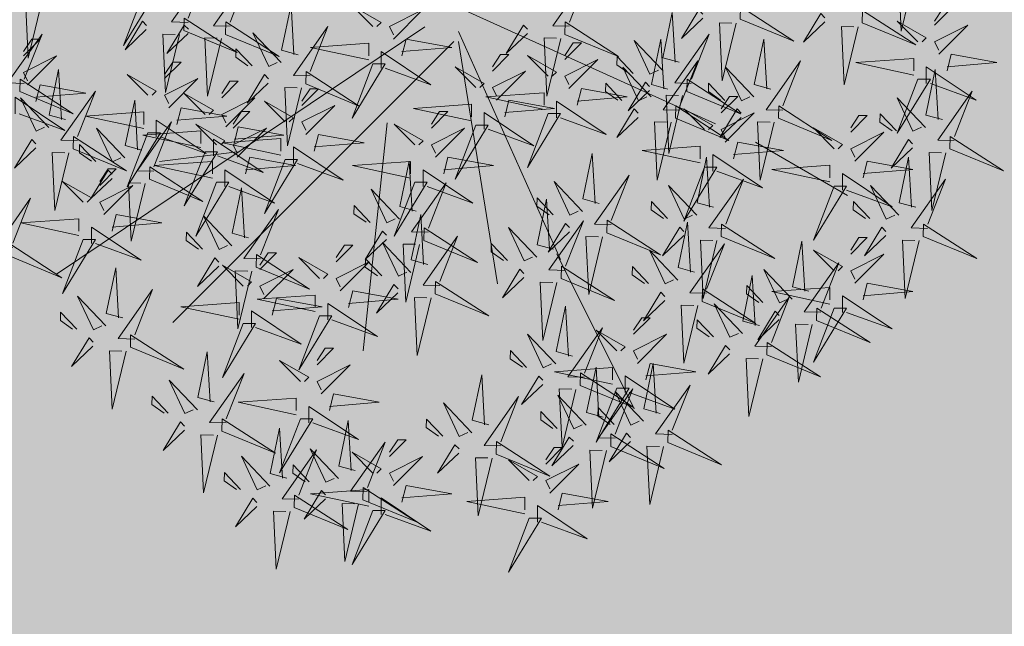
# Model space of a CAD drawing. Units: inches. Extents: x 1704 to 6393, y -157 to 1172.
# Tile 108 of 122: x 2688 to 2716, y 972 to 989. Entities that reach past the tile are written whole.
import ezdxf

# ---------------------------------------------------------------- set-up
doc = ezdxf.new("R2010")
doc.units = ezdxf.units.IN
doc.header["$MEASUREMENT"] = 0
doc.layers.add('A-ANNO-DIMS', color=7, linetype='Continuous', lineweight=13)
doc.layers.add('L-shrub', color=74, linetype='Continuous', lineweight=18)
doc.layers.add('L-HRDS-PATT', color=9, linetype='Continuous', lineweight=13, true_color=0xc5c1ba)
doc.styles.get("Standard").update_dxf_attribs({"font": 'arial.ttf'})
doc.dimstyles.get("Standard").update_dxf_attribs({"dimtxt": 6, "dimasz": 2, "dimexe": 0.18, "dimexo": 0.0625, "dimgap": 0.09, "dimtad": 0, "dimtih": 1, "dimtoh": 1, "dimdec": 1, "dimzin": 0, "dimdsep": 46, "dimlunit": 3, "dimtxsty": 'Standard', "dimblk": 'ARCHTICK', "dimcen": 0.09, "dimadec": 0, "dimazin": 0, "dimtfac": 1, "dimtdec": 1, "dimtofl": 0, "dimtmove": 0, "dimatfit": 3, "dimfxl": 1, "dimtolj": 1, "dimtzin": 0, "dimarcsym": 0})

# ---------------------------------------------------------------- blocks, each defined once
blk = doc.blocks.new('shrub3')
for p, q in [((68.94, 162.35), (98.58, 213.48)), ((-5.99, -2.5), (58.67, 140.12)), ((130.91, 52.02), (217.13, 95.08)), ((7.48, -2.5), (134.11, 54.01)), ((12.87, -2.5), (147.58, 19.03)), ((12.87, -5.19), (169.14, -161.27)), ((4.78, -21.34), (142.19, -225.85)), ((58.17, -42.16), (184.8, -55.61)), ((74.33, -125.58), (79.72, -168.64))]:
    blk.add_line(p, q)
for points in [[(29.32, 268.76), (20.08, 271.07), (24.7, 296.43), (27.01, 268.76)], [(72.58, 270.39), (84.86, 300.11), (65.67, 270.57), (72.58, 270.39)], [(36.24, 257.23), (27.01, 257.23), (45.48, 284.9), (36.24, 259.54)], [(121.34, 255.57), (133.62, 285.29), (114.43, 255.75), (121.34, 255.57)], [(20.08, 264.15), (3.92, 280.29), (13.16, 261.85), (17.78, 264.15)], [(68.03, 272.82), (67.8, 263.59), (40.6, 282.74), (65.73, 272.87)], [(3.92, 261.85), (-5.31, 271.07), (-5.31, 266.46), (1.62, 261.85)], [(74.83, 268.03), (106.93, 260.3), (74.6, 258.8), (74.77, 265.72)], [(56.33, 266.18), (53.8, 257.01), (28.56, 262.26), (56.27, 263.87)], [(116.79, 258), (116.56, 248.76), (89.36, 267.92), (114.49, 258.05)], [(13.16, 252.62), (1.62, 241.09), (10.85, 257.23), (13.16, 254.93)], [(33.94, 252.62), (63.95, 241.09), (33.94, 259.54), (33.94, 252.62)], [(60.71, 256.84), (44.17, 241.08), (62.84, 249.85), (60.65, 254.53)], [(123.59, 253.21), (155.69, 245.48), (123.36, 243.97), (123.53, 250.9)], [(-24.81, 251.09), (7.29, 243.36), (-25.04, 241.86), (-24.87, 248.78)], [(2.62, 221.69), (14.9, 251.41), (-4.29, 221.87), (2.62, 221.69)], [(31.63, 250.32), (24.7, 218.04), (22.39, 250.32), (29.32, 250.32)], [(72.06, 249.62), (83.3, 237.79), (67.4, 247.43), (69.76, 249.68)], [(105.09, 251.36), (102.56, 242.19), (77.32, 247.44), (105.04, 249.05)], [(88.68, 222.18), (79.44, 224.49), (84.06, 249.85), (86.37, 222.18)], [(156.52, 222.18), (147.29, 224.49), (151.9, 249.85), (154.21, 222.18)], [(109.47, 242.01), (92.93, 226.26), (111.6, 235.03), (109.41, 239.71)], [(62.61, 240.62), (53.16, 231.62), (57.77, 231.51), (62.55, 238.31)], [(95.61, 210.65), (86.37, 210.65), (104.84, 238.32), (95.61, 212.96)], [(163.45, 210.65), (154.21, 210.65), (172.68, 238.32), (163.45, 212.96)], [(79.44, 217.57), (63.28, 233.71), (72.52, 215.26), (77.14, 217.57)], [(120.82, 234.8), (132.06, 222.97), (116.16, 232.61), (118.52, 234.86)], [(147.29, 217.57), (131.13, 233.71), (140.36, 215.26), (144.98, 217.57)], [(63.28, 215.26), (54.05, 224.49), (54.05, 219.87), (60.98, 215.26)], [(111.37, 225.8), (101.92, 216.8), (106.53, 216.68), (111.31, 223.49)], [(131.13, 215.26), (121.89, 224.49), (121.89, 219.87), (128.82, 215.26)], [(167.98, 196.29), (180.26, 226), (161.07, 196.46), (167.98, 196.29)], [(4.87, 219.33), (36.97, 211.6), (4.64, 210.1), (4.81, 217.02)], [(72.52, 206.04), (60.98, 194.51), (70.21, 210.65), (72.52, 208.35)], [(93.3, 206.04), (123.31, 194.51), (93.3, 212.96), (93.3, 206.04)], [(140.36, 206.04), (128.82, 194.51), (138.05, 210.65), (140.36, 208.35)], [(163.43, 198.71), (163.2, 189.48), (136, 208.63), (161.13, 198.77)], [(161.14, 206.04), (191.15, 194.51), (161.14, 212.96), (161.14, 206.04)], [(55.62, 175.11), (67.9, 204.83), (48.71, 175.28), (55.62, 175.11)], [(90.99, 203.73), (84.06, 171.45), (81.75, 203.73), (88.68, 203.73)], [(158.83, 203.73), (151.9, 171.45), (149.59, 203.73), (156.52, 203.73)], [(2.1, 200.92), (13.34, 189.09), (-2.56, 198.73), (-0.2, 200.98)], [(187.06, 168.76), (199.34, 198.47), (180.15, 168.93), (187.06, 168.76)], [(151.73, 192.07), (149.2, 182.9), (123.96, 188.15), (151.68, 189.77)], [(170.23, 193.92), (202.33, 186.19), (170, 184.69), (170.17, 191.61)], [(51.07, 177.53), (50.84, 168.3), (23.64, 187.46), (48.77, 177.59)], [(0.5, 153.94), (12.78, 183.65), (-6.41, 154.11), (0.5, 153.94)], [(156.11, 182.73), (139.57, 166.97), (158.24, 175.74), (156.05, 180.42)], [(182.51, 171.18), (182.28, 161.95), (155.08, 181.11), (180.21, 171.24)], [(78.08, 150.19), (68.84, 152.49), (73.46, 177.86), (75.77, 150.19)], [(167.46, 175.51), (178.7, 163.69), (162.8, 173.32), (165.16, 175.57)], [(39.37, 170.9), (36.84, 161.73), (11.6, 166.98), (39.31, 168.59)], [(57.87, 172.75), (89.97, 165.01), (57.64, 163.51), (57.81, 170.44)], [(121.34, 143.35), (133.62, 173.06), (114.43, 143.52), (121.34, 143.35)], [(85.01, 138.66), (75.77, 138.66), (94.24, 166.33), (85.01, 140.97)], [(170.81, 164.55), (168.28, 155.37), (143.04, 160.62), (170.76, 162.24)], [(158.01, 166.51), (148.56, 157.51), (153.17, 157.4), (157.96, 164.21)], [(189.31, 166.39), (221.41, 158.66), (189.08, 157.16), (189.25, 164.09)], [(43.75, 161.55), (27.21, 145.8), (45.88, 154.57), (43.69, 159.24)], [(68.84, 145.58), (52.68, 161.72), (61.92, 143.27), (66.54, 145.58)], [(157.38, 132.76), (169.66, 162.48), (150.47, 132.94), (157.38, 132.76)], [(40.78, 124.29), (53.06, 154.01), (33.87, 124.47), (40.78, 124.29)], [(55.1, 154.34), (66.34, 142.51), (50.44, 152.15), (52.8, 154.4)], [(116.79, 145.77), (116.56, 136.54), (89.36, 155.7), (114.49, 145.83)], [(175.19, 155.2), (158.65, 139.45), (177.32, 148.22), (175.13, 152.89)], [(2.75, 151.57), (34.85, 143.84), (2.52, 142.34), (2.69, 149.26)], [(52.68, 143.27), (43.45, 152.49), (43.45, 147.88), (50.38, 143.27)], [(186.54, 147.99), (197.78, 136.16), (181.88, 145.8), (184.24, 148.05)], [(45.65, 145.34), (36.2, 136.34), (40.81, 136.22), (45.59, 143.03)], [(55.62, 117.94), (67.9, 147.66), (48.71, 118.11), (55.62, 117.94)], [(152.83, 135.19), (152.6, 125.95), (125.4, 145.11), (150.53, 135.24)], [(235.82, 113.71), (248.1, 143.42), (228.91, 113.88), (235.82, 113.71)], [(61.92, 134.05), (50.38, 122.52), (59.61, 138.66), (61.92, 136.35)], [(105.09, 139.14), (102.56, 129.96), (77.32, 135.21), (105.04, 136.83)], [(82.7, 134.05), (112.71, 122.52), (82.7, 140.97), (82.7, 134.05)], [(123.59, 140.98), (155.69, 133.25), (123.36, 131.75), (123.53, 138.68)], [(177.09, 138.99), (167.64, 129.99), (172.25, 129.87), (177.04, 136.68)], [(-0.02, 133.17), (11.22, 121.34), (-4.68, 130.97), (-2.32, 133.22)], [(36.23, 126.72), (36, 117.49), (8.8, 136.64), (33.93, 126.77)], [(80.39, 131.74), (73.46, 99.46), (71.15, 131.74), (78.08, 131.74)], [(51.07, 120.36), (50.84, 111.13), (23.64, 130.29), (48.77, 120.42)], [(109.47, 129.79), (92.93, 114.04), (111.6, 122.81), (109.41, 127.48)], [(141.13, 128.55), (138.6, 119.38), (113.36, 124.63), (141.08, 126.24)], [(159.63, 130.4), (191.73, 122.67), (159.4, 121.17), (159.57, 128.09)], [(201.04, 101.49), (191.81, 103.79), (196.42, 129.16), (198.73, 101.49)], [(231.27, 116.13), (231.04, 106.9), (203.84, 126.05), (228.97, 116.19)], [(43.03, 121.93), (75.13, 114.2), (42.8, 112.7), (42.97, 119.62)], [(120.82, 122.58), (132.06, 110.75), (116.16, 120.39), (118.52, 122.64)], [(24.53, 120.08), (22, 110.91), (-3.24, 116.16), (24.47, 117.77)], [(57.87, 115.58), (89.97, 107.84), (57.64, 106.34), (57.81, 113.27)], [(145.51, 119.2), (128.97, 103.45), (147.64, 112.22), (145.45, 116.9)], [(207.97, 89.96), (198.73, 89.96), (217.2, 117.63), (207.97, 92.27)], [(39.37, 113.73), (36.84, 104.56), (11.6, 109.81), (39.31, 111.42)], [(28.91, 110.73), (12.37, 94.98), (31.04, 103.75), (28.85, 108.43)], [(111.37, 113.58), (101.92, 104.58), (106.53, 104.46), (111.31, 111.27)], [(119.22, 79.83), (131.5, 109.54), (112.31, 80), (119.22, 79.83)], [(156.86, 111.99), (168.1, 100.16), (152.2, 109.8), (154.56, 112.05)], [(191.81, 96.88), (175.65, 113.02), (184.88, 94.57), (189.5, 96.88)], [(219.57, 109.49), (217.04, 100.32), (191.8, 105.57), (219.52, 107.19)], [(237.94, 81.95), (250.22, 111.66), (231.03, 82.12), (237.94, 81.95)], [(238.07, 111.34), (270.17, 103.61), (237.84, 102.11), (238.01, 109.03)], [(43.75, 104.38), (27.21, 88.63), (45.88, 97.4), (43.69, 102.07)], [(40.26, 103.52), (51.5, 91.69), (35.6, 101.33), (37.96, 103.58)], [(147.41, 102.99), (137.96, 93.99), (142.57, 93.88), (147.36, 100.68)], [(175.65, 94.57), (166.41, 103.79), (166.41, 99.18), (173.34, 94.57)], [(223.95, 100.15), (207.41, 84.4), (226.08, 93.17), (223.89, 97.84)], [(30.81, 94.52), (21.36, 85.52), (25.97, 85.41), (30.75, 92.21)], [(55.1, 97.17), (66.34, 85.34), (50.44, 94.98), (52.8, 97.23)], [(204.02, 65.01), (216.3, 94.72), (197.11, 65.18), (204.02, 65.01)], [(233.39, 84.37), (233.16, 75.14), (205.96, 94.29), (231.09, 84.43)], [(235.3, 92.94), (246.54, 81.11), (230.64, 90.74), (233, 92.99)], [(45.65, 88.17), (36.2, 79.17), (40.81, 79.05), (45.59, 85.86)], [(48.4, 63.38), (39.16, 65.68), (43.78, 91.04), (46.09, 63.38)], [(114.67, 82.25), (114.44, 73.02), (87.24, 92.18), (112.37, 82.31)], [(184.88, 85.35), (173.34, 73.82), (182.57, 89.96), (184.88, 87.65)], [(205.66, 85.35), (235.67, 73.82), (205.66, 92.27), (205.66, 85.35)], [(8.98, 56.54), (21.26, 86.25), (2.07, 56.71), (8.98, 56.54)], [(144.66, 54.42), (156.94, 84.13), (137.75, 54.59), (144.66, 54.42)], [(203.35, 83.04), (196.42, 50.76), (194.11, 83.04), (201.04, 83.04)], [(225.85, 83.93), (216.4, 74.93), (221.01, 74.82), (225.8, 81.63)], [(55.33, 51.85), (46.09, 51.85), (64.56, 79.52), (55.33, 54.15)], [(121.47, 77.46), (153.57, 69.73), (121.24, 68.23), (121.41, 75.15)], [(199.47, 67.43), (199.24, 58.2), (172.04, 77.35), (197.17, 67.49)], [(221.69, 77.73), (219.16, 68.56), (193.92, 73.81), (221.64, 75.43)], [(240.19, 79.58), (272.29, 71.85), (239.96, 70.35), (240.13, 77.27)], [(273.12, 52.79), (263.89, 55.09), (268.5, 80.46), (270.81, 52.79)], [(39.16, 58.76), (23, 74.9), (32.24, 56.46), (36.86, 58.76)], [(102.97, 75.62), (100.44, 66.44), (75.2, 71.69), (102.92, 73.31)], [(4.43, 58.96), (4.2, 49.73), (-23, 68.88), (2.13, 59.02)], [(23, 56.46), (13.77, 65.68), (13.77, 61.07), (20.7, 56.46)], [(107.35, 66.27), (90.81, 50.52), (109.48, 59.29), (107.29, 63.96)], [(140.11, 56.84), (139.88, 47.61), (112.68, 66.77), (137.81, 56.9)], [(226.07, 68.39), (209.53, 52.64), (228.2, 61.41), (226.01, 66.08)], [(280.05, 41.26), (270.81, 41.26), (289.28, 68.93), (280.05, 43.57)], [(187.77, 60.79), (185.24, 51.62), (160, 56.87), (187.72, 58.49)], [(206.27, 62.64), (238.37, 54.91), (206.04, 53.41), (206.21, 60.33)], [(237.42, 61.17), (248.66, 49.35), (232.76, 58.98), (235.12, 61.23)], [(263.89, 48.18), (247.73, 64.32), (256.96, 45.87), (261.58, 48.18)], [(118.7, 59.06), (129.94, 47.23), (114.04, 56.86), (116.4, 59.12)], [(247.73, 45.87), (238.49, 55.09), (238.49, 50.48), (245.42, 45.87)], [(11.23, 54.17), (43.33, 46.44), (11, 44.94), (11.17, 51.86)], [(32.24, 47.24), (20.7, 35.71), (29.93, 51.85), (32.24, 49.54)], [(54.76, 23.15), (45.52, 25.45), (50.14, 50.81), (52.45, 23.15)], [(53.02, 47.24), (83.03, 35.71), (53.02, 54.15), (53.02, 47.24)], [(109.25, 50.06), (99.8, 41.06), (104.41, 40.94), (109.19, 47.75)], [(128.41, 50.21), (125.88, 41.03), (100.64, 46.28), (128.36, 47.9)], [(146.91, 52.05), (179.01, 44.32), (146.68, 42.82), (146.85, 49.75)], [(192.15, 51.45), (175.61, 35.7), (194.28, 44.47), (192.09, 49.14)], [(227.97, 52.17), (218.52, 43.17), (223.13, 43.06), (227.92, 49.87)], [(50.71, 44.93), (43.78, 12.65), (41.47, 44.93), (48.4, 44.93)], [(203.5, 44.24), (214.74, 32.41), (198.84, 42.04), (201.2, 44.29)], [(242.18, 18.42), (254.46, 48.14), (235.27, 18.6), (242.18, 18.42)], [(61.69, 11.62), (52.45, 11.62), (70.92, 39.29), (61.69, 13.92)], [(132.79, 40.86), (116.25, 25.11), (134.92, 33.88), (132.73, 38.55)], [(256.96, 36.65), (245.42, 25.12), (254.65, 41.26), (256.96, 38.95)], [(277.74, 36.65), (307.75, 25.12), (277.74, 43.57), (277.74, 36.65)], [(8.46, 35.77), (19.7, 23.94), (3.8, 33.57), (6.16, 35.82)], [(45.52, 18.53), (29.36, 34.67), (38.6, 16.23), (43.22, 18.53)], [(144.14, 33.65), (155.38, 21.82), (139.48, 31.46), (141.84, 33.71)], [(194.05, 35.23), (184.6, 26.23), (189.21, 26.12), (194, 32.93)], [(275.43, 34.34), (268.5, 2.06), (266.19, 34.34), (273.12, 34.34)], [(237.63, 20.85), (237.4, 11.62), (210.2, 30.77), (235.33, 20.91)], [(29.36, 16.23), (20.13, 25.45), (20.13, 20.84), (27.06, 16.23)], [(134.69, 24.65), (125.24, 15.65), (129.85, 15.53), (134.63, 22.34)], [(86.56, -10.73), (77.32, -8.43), (81.94, 16.94), (84.25, -10.73)], [(38.6, 7), (27.06, -4.52), (36.29, 11.62), (38.6, 9.31)], [(59.38, 7), (89.39, -4.52), (59.38, 13.92), (59.38, 7)], [(153.14, -15.45), (165.42, 14.26), (146.23, -15.28), (153.14, -15.45)], [(225.93, 14.21), (223.4, 5.04), (198.16, 10.29), (225.88, 11.9)], [(244.43, 16.06), (276.53, 8.33), (244.2, 6.83), (244.37, 13.75)], [(123.46, -21.81), (135.74, 7.91), (116.55, -21.63), (123.46, -21.81)], [(57.07, 4.7), (50.14, -27.58), (47.83, 4.7), (54.76, 4.7)], [(77.32, -15.34), (61.16, 0.8), (70.4, -17.65), (75.02, -15.34)], [(93.49, -22.26), (84.25, -22.26), (102.72, 5.41), (93.49, -19.96)], [(230.31, 4.87), (213.77, -10.89), (232.44, -2.12), (230.25, 2.56)], [(148.59, -13.03), (148.36, -22.26), (121.16, -3.11), (146.29, -12.97)], [(241.66, -2.35), (252.9, -14.18), (237, -4.54), (239.36, -2.29)], [(20.84, -34.02), (11.6, -31.72), (16.22, -6.36), (18.53, -34.02)], [(61.16, -17.65), (51.93, -8.43), (51.93, -13.04), (58.86, -17.65)], [(118.91, -19.38), (118.68, -28.61), (91.48, -9.46), (116.61, -19.33)], [(268.88, -34.02), (259.65, -31.72), (264.26, -6.36), (266.57, -34.02)], [(232.21, -11.35), (222.76, -20.35), (227.37, -20.46), (232.16, -13.66)], [(27.76, -45.55), (18.53, -45.55), (37, -17.88), (27.76, -43.25)], [(91.18, -26.87), (121.19, -38.4), (91.18, -19.96), (91.18, -26.87)], [(136.89, -19.67), (134.36, -28.84), (109.12, -23.59), (136.84, -21.97)], [(155.39, -17.82), (187.49, -25.55), (155.16, -27.05), (155.33, -20.13)], [(275.81, -45.55), (266.57, -45.55), (285.04, -17.88), (275.81, -43.25)], [(11.6, -38.64), (-4.56, -22.5), (4.68, -40.94), (9.3, -38.64)], [(70.4, -26.87), (58.86, -38.4), (68.09, -22.26), (70.4, -24.57)], [(107.21, -26.02), (104.68, -35.19), (79.44, -29.94), (107.16, -28.33)], [(125.71, -24.17), (157.81, -31.9), (125.48, -33.4), (125.65, -26.48)], [(259.65, -38.64), (243.49, -22.5), (252.72, -40.94), (257.34, -38.64)], [(267.62, -55.68), (279.9, -25.97), (260.71, -55.51), (267.62, -55.68)], [(88.87, -29.18), (81.94, -61.46), (79.63, -29.18), (86.56, -29.18)], [(141.27, -29.01), (124.73, -44.76), (143.4, -35.99), (141.21, -31.32)], [(243.49, -40.94), (234.25, -31.72), (234.25, -36.33), (241.18, -40.94)], [(111.59, -35.37), (95.05, -51.12), (113.72, -42.35), (111.53, -37.67)], [(152.62, -36.23), (163.86, -48.05), (147.96, -38.42), (150.32, -36.17)], [(160.76, -63.67), (151.53, -61.36), (156.14, -36), (158.45, -63.67)], [(25.46, -50.16), (55.47, -61.69), (25.46, -43.25), (25.46, -50.16)], [(122.94, -42.58), (134.18, -54.41), (118.28, -44.77), (120.64, -42.52)], [(263.07, -53.26), (262.84, -62.49), (235.64, -43.34), (260.77, -53.2)], [(273.5, -50.16), (303.51, -61.69), (273.5, -43.25), (273.5, -50.16)], [(4.68, -50.16), (-6.86, -61.69), (2.37, -45.55), (4.68, -47.86)], [(143.17, -45.23), (133.72, -54.23), (138.33, -54.34), (143.12, -47.53)], [(167.69, -75.2), (158.45, -75.2), (176.92, -47.53), (167.69, -72.89)], [(218, -74.25), (208.77, -71.95), (213.38, -46.59), (215.69, -74.25)], [(252.72, -50.16), (241.18, -61.69), (250.41, -45.55), (252.72, -47.86)], [(23.15, -52.47), (16.22, -84.75), (13.91, -52.47), (20.84, -52.47)], [(113.49, -51.58), (104.04, -60.58), (108.65, -60.69), (113.43, -53.89)], [(151.53, -68.28), (135.37, -52.14), (144.6, -70.59), (149.22, -68.28)], [(271.19, -52.47), (264.26, -84.75), (261.95, -52.47), (268.88, -52.47)], [(36.54, -87.45), (48.82, -57.73), (29.63, -87.27), (36.54, -87.45)], [(73.84, -82.72), (64.6, -80.42), (69.22, -55.06), (71.53, -82.72)], [(224.93, -85.78), (215.69, -85.78), (234.16, -58.11), (224.93, -83.48)], [(251.37, -59.9), (248.84, -69.07), (223.6, -63.82), (251.32, -62.2)], [(269.87, -58.05), (301.97, -65.78), (269.64, -67.28), (269.81, -60.36)], [(135.37, -70.59), (126.13, -61.36), (126.13, -65.97), (133.06, -70.59)], [(208.77, -78.87), (192.61, -62.73), (201.84, -81.17), (206.46, -78.87)], [(271.86, -93.8), (284.14, -64.08), (264.95, -93.62), (271.86, -93.8)], [(80.77, -94.25), (71.53, -94.25), (90, -66.58), (80.77, -91.95)], [(255.75, -69.24), (239.21, -85), (257.88, -76.23), (255.7, -71.55)], [(31.99, -85.02), (31.76, -94.25), (4.56, -75.1), (29.69, -84.96)], [(64.6, -87.34), (48.44, -71.2), (57.68, -89.64), (62.3, -87.34)], [(144.6, -79.81), (133.06, -91.34), (142.29, -75.2), (144.6, -77.5)], [(165.38, -79.81), (195.39, -91.34), (165.38, -72.89), (165.38, -79.81)], [(192.61, -81.17), (183.37, -71.95), (183.37, -76.56), (190.3, -81.17)], [(267.1, -76.46), (278.34, -88.28), (262.44, -78.65), (264.8, -76.4)], [(48.44, -89.64), (39.21, -80.42), (39.21, -85.03), (46.14, -89.64)], [(165, -106.02), (155.77, -103.71), (160.38, -78.35), (162.69, -106.02)], [(267.31, -91.37), (267.08, -100.61), (239.88, -81.45), (265.01, -91.32)], [(138.3, -114.97), (150.58, -85.26), (131.39, -114.8), (138.3, -114.97)], [(163.07, -82.11), (156.14, -114.39), (153.83, -82.11), (160.76, -82.11)], [(201.84, -90.4), (190.3, -101.92), (199.53, -85.78), (201.84, -88.09)], [(222.62, -90.4), (252.63, -101.92), (222.62, -83.48), (222.62, -90.4)], [(257.65, -85.46), (248.2, -94.46), (252.81, -94.57), (257.6, -87.76)], [(20.29, -91.66), (17.76, -100.83), (-7.48, -95.58), (20.23, -93.97)], [(38.79, -89.81), (70.89, -97.54), (38.56, -99.04), (38.73, -92.12)], [(78.46, -98.86), (108.47, -110.39), (78.46, -91.95), (78.46, -98.86)], [(171.93, -117.54), (162.69, -117.54), (181.16, -89.88), (171.93, -115.24)], [(220.31, -92.7), (213.38, -124.98), (211.07, -92.7), (218, -92.7)], [(57.68, -98.86), (46.14, -110.39), (55.37, -94.25), (57.68, -96.56)], [(86.56, -120.84), (77.32, -118.53), (81.94, -93.17), (84.25, -120.84)], [(155.77, -110.63), (139.61, -94.49), (148.84, -112.93), (153.46, -110.63)], [(255.61, -98.01), (253.08, -107.18), (227.84, -101.93), (255.56, -100.32)], [(274.11, -96.16), (306.21, -103.89), (273.88, -105.4), (274.05, -98.47)], [(8.98, -131.91), (21.26, -102.2), (2.07, -131.74), (8.98, -131.91)], [(24.67, -101), (8.13, -116.76), (26.8, -107.99), (24.61, -103.31)], [(69.6, -127.19), (60.36, -124.88), (64.98, -99.52), (67.29, -127.19)], [(76.15, -101.17), (69.22, -133.45), (66.91, -101.17), (73.84, -101.17)], [(133.75, -112.55), (133.52, -121.78), (106.32, -102.62), (131.45, -112.49)], [(139.61, -112.93), (130.37, -103.71), (130.37, -108.32), (137.3, -112.93)], [(36.02, -108.22), (47.26, -120.04), (31.36, -110.41), (33.72, -108.16)], [(77.32, -125.45), (61.16, -109.31), (70.4, -127.75), (75.02, -125.45)], [(93.49, -132.37), (84.25, -132.37), (102.72, -104.7), (93.49, -130.06)], [(229.46, -134.03), (241.74, -104.31), (222.55, -133.86), (229.46, -134.03)], [(259.99, -107.36), (243.45, -123.11), (262.12, -114.34), (259.94, -109.66)], [(76.53, -138.72), (67.29, -138.72), (85.76, -111.05), (76.53, -136.41)], [(271.34, -114.57), (282.58, -126.4), (266.68, -116.76), (269.04, -114.51)], [(4.43, -129.49), (4.2, -138.72), (-23, -119.56), (2.13, -129.43)], [(26.57, -117.22), (17.12, -126.22), (21.73, -126.33), (26.51, -119.53)], [(60.36, -131.8), (44.2, -115.66), (53.44, -134.11), (58.06, -131.8)], [(61.16, -127.75), (51.93, -118.53), (51.93, -123.14), (58.86, -127.75)], [(122.05, -119.18), (119.52, -128.36), (94.28, -123.11), (122, -121.49)], [(148.84, -122.16), (137.3, -133.69), (146.53, -117.54), (148.84, -119.85)], [(140.55, -117.34), (172.65, -125.07), (140.32, -126.57), (140.49, -119.65)], [(169.62, -122.16), (199.63, -133.69), (169.62, -115.24), (169.62, -122.16)], [(6.86, -155.2), (19.14, -125.49), (-0.05, -155.03), (6.86, -155.2)], [(44.2, -134.11), (34.97, -124.88), (34.97, -129.5), (41.9, -134.11)], [(167.31, -124.46), (160.38, -156.74), (158.07, -124.46), (165, -124.46)], [(224.91, -131.61), (224.68, -140.84), (197.48, -121.68), (222.61, -131.55)], [(261.89, -123.57), (252.44, -132.57), (257.05, -132.69), (261.84, -125.88)], [(91.18, -136.98), (121.19, -148.51), (91.18, -130.06), (91.18, -136.98)], [(126.43, -128.53), (109.89, -144.28), (128.56, -135.51), (126.37, -130.84)], [(11.23, -134.28), (43.33, -142.01), (11, -143.51), (11.17, -136.58)], [(59, -158.95), (49.76, -156.64), (54.38, -131.28), (56.69, -158.95)], [(70.4, -136.98), (58.86, -148.51), (68.09, -132.37), (70.4, -134.67)], [(74.22, -143.33), (104.23, -154.86), (74.22, -136.41), (74.22, -143.33)], [(137.78, -135.74), (149.02, -147.57), (133.12, -137.94), (135.48, -135.69)], [(231.71, -136.39), (263.81, -144.13), (231.48, -145.63), (231.65, -138.7)], [(53.44, -143.33), (41.9, -154.86), (51.13, -138.72), (53.44, -141.02)], [(88.87, -139.28), (81.94, -171.56), (79.63, -139.28), (86.56, -139.28)], [(213.21, -138.24), (210.68, -147.41), (185.44, -142.16), (213.16, -140.55)], [(2.31, -152.78), (2.08, -162.01), (-25.12, -142.86), (0.01, -152.72)], [(49.76, -163.56), (33.6, -147.42), (42.84, -165.87), (47.46, -163.56)], [(65.93, -170.48), (56.69, -170.48), (75.16, -142.81), (65.93, -168.17)], [(71.91, -145.64), (64.98, -177.92), (62.67, -145.64), (69.6, -145.64)], [(89.54, -174.26), (101.82, -144.54), (82.63, -174.09), (89.54, -174.26)], [(128.33, -144.74), (118.88, -153.74), (123.49, -153.86), (128.27, -147.05)], [(217.59, -147.59), (201.05, -163.34), (219.72, -154.57), (217.53, -149.9)], [(8.46, -152.68), (19.7, -164.51), (3.8, -154.87), (6.16, -152.62)], [(9.11, -157.57), (41.21, -165.3), (8.88, -166.8), (9.05, -159.88)], [(33.6, -165.87), (24.37, -156.64), (24.37, -161.26), (31.3, -165.87)], [(182.82, -184.85), (195.1, -155.13), (175.91, -184.67), (182.82, -184.85)], [(228.94, -154.8), (240.18, -166.63), (224.28, -156.99), (226.64, -154.74)], [(84.99, -171.84), (84.76, -181.07), (57.56, -161.91), (82.69, -171.78)], [(219.49, -163.8), (210.04, -172.8), (214.65, -172.92), (219.44, -166.11)], [(63.62, -175.09), (93.63, -186.62), (63.62, -168.17), (63.62, -175.09)], [(118.36, -194.95), (109.13, -192.64), (113.74, -167.28), (116.05, -194.95)], [(-14.82, -177.21), (15.19, -188.74), (-14.82, -170.29), (-14.82, -177.21)], [(42.84, -175.09), (31.3, -186.62), (40.53, -170.48), (42.84, -172.79)], [(178.27, -182.42), (178.04, -191.65), (150.84, -172.5), (175.97, -182.36)], [(6.34, -175.97), (17.58, -187.8), (1.68, -178.17), (4.04, -175.92)], [(73.29, -178.47), (70.76, -187.64), (45.52, -182.39), (73.23, -180.78)], [(61.31, -177.4), (54.38, -209.68), (52.07, -177.4), (59, -177.4)], [(91.79, -176.62), (123.89, -184.36), (91.56, -185.86), (91.73, -178.93)], [(125.29, -206.48), (116.05, -206.48), (134.52, -178.81), (125.29, -204.17)], [(109.13, -199.56), (92.96, -183.42), (102.2, -201.86), (106.82, -199.56)], [(77.67, -187.82), (61.13, -203.57), (79.8, -194.8), (77.61, -190.13)], [(72.58, -216.61), (84.86, -186.89), (65.67, -216.43), (72.58, -216.61)], [(166.57, -189.06), (164.04, -198.23), (138.8, -192.98), (166.52, -191.37)], [(185.07, -187.21), (217.17, -194.94), (184.84, -196.44), (185.01, -189.52)], [(92.96, -201.86), (83.73, -192.64), (83.73, -197.25), (90.66, -201.86)], [(89.02, -195.03), (100.26, -206.86), (84.36, -197.22), (86.72, -194.97)], [(170.95, -198.4), (154.41, -214.16), (173.08, -205.39), (170.89, -200.71)], [(68.03, -214.18), (67.8, -223.42), (40.6, -204.26), (65.73, -214.13)], [(79.57, -204.03), (70.12, -213.03), (74.73, -213.15), (79.51, -206.34)], [(102.2, -211.09), (90.66, -222.62), (99.89, -206.48), (102.2, -208.78)], [(122.98, -211.09), (152.99, -222.62), (122.98, -204.17), (122.98, -211.09)], [(182.3, -205.62), (193.54, -217.44), (177.64, -207.81), (180, -205.56)], [(46.28, -237.29), (37.04, -234.99), (41.66, -209.63), (43.97, -237.29)], [(40.78, -246.25), (53.06, -216.54), (33.87, -246.08), (40.78, -246.25)], [(120.67, -213.39), (113.74, -245.67), (111.43, -213.39), (118.36, -213.39)], [(172.85, -214.62), (163.4, -223.62), (168.01, -223.73), (172.8, -216.93)], [(56.33, -220.82), (53.8, -229.99), (28.56, -224.74), (56.27, -223.13)], [(53.21, -248.82), (43.97, -248.82), (62.44, -221.15), (53.21, -246.52)], [(74.83, -218.97), (106.93, -226.7), (74.6, -228.2), (74.77, -221.28)], [(131.94, -252.6), (144.22, -222.89), (125.03, -252.43), (131.94, -252.6)], [(37.04, -241.91), (20.88, -225.77), (30.12, -244.21), (34.74, -241.91)], [(-9.97, -233.79), (22.13, -241.53), (-10.2, -243.03), (-10.03, -236.1)], [(36.23, -243.83), (36, -253.06), (8.8, -233.9), (33.93, -243.77)], [(20.88, -244.21), (11.65, -234.99), (11.65, -239.6), (18.58, -244.21)], [(60.71, -230.17), (44.17, -245.92), (62.84, -237.15), (60.65, -232.47)], [(72.06, -237.38), (83.3, -249.21), (67.4, -239.57), (69.76, -237.32)], [(127.39, -250.18), (127.16, -259.41), (99.96, -240.26), (125.09, -250.12)]]:
    blk.add_lwpolyline(points)
blk = doc.blocks.new('_ArchTick')
at = {"color": 0, "linetype": 'ByBlock', "const_width": 0.15}
blk.add_lwpolyline([(-0.5, -0.5), (0.5, 0.5)], dxfattribs=at)
blk = doc.blocks.new('*D95')
at = {"layer": 'A-ANNO-DIMS', "color": 0, "lineweight": -2, "transparency": 16777216}
for p, q in [((2605.349, 895.275), (2605.349, 1105.287)), ((2723.349, 895.275), (2723.349, 1105.287)), ((2605.349, 1105.107), (2657.907, 1105.107)), ((2723.349, 1105.107), (2670.791, 1105.107))]:
    blk.add_line(p, q, dxfattribs=at)
at = {"layer": 'Defpoints', "color": 0, "lineweight": -3, "transparency": 16777216}
for p in [(2723.349, 1105.107), (2605.349, 895.213), (2723.349, 895.213)]:
    blk.add_point(p, dxfattribs=at)
at = {"layer": 'A-ANNO-DIMS', "color": 0, "lineweight": -2, "transparency": 16777216, "xscale": 2, "yscale": 2, "zscale": 2, "rotation": 180}
blk.add_blockref('_ArchTick', (2605.349, 1105.107), dxfattribs=at)
at = {"layer": 'A-ANNO-DIMS', "color": 0, "lineweight": -2, "transparency": 16777216, "xscale": 2, "yscale": 2, "zscale": 2}
blk.add_blockref('_ArchTick', (2723.349, 1105.107), dxfattribs=at)
at = {"layer": 'A-ANNO-DIMS', "color": 0, "transparency": 16777216, "insert": (2664.349, 1105.107), "char_height": 6, "attachment_point": 5}
blk.add_mtext('\\A1;118', dxfattribs=at)

msp = doc.modelspace()

# ---------------------------------------------------------------- hatches: boundary and pattern name
at = {"layer": 'L-HRDS-PATT', "transparency": 33554661}
h = msp.add_hatch(color=256, dxfattribs=at)
h.dxf.hatch_style = 1
h.paths.add_polyline_path([(2719.349, 1033.213), (2664.349, 1033.213), (2664.349, 895.213), (2719.349, 895.213)])
h.paths.add_polyline_path([(2719.349, 895.213), (2664.349, 895.213), (2605.349, 895.213), (2605.349, 872.213), (2719.349, 872.213)])
h.paths.add_polyline_path([(2719.349, 872.213), (2605.349, 872.213), (2605.349, 854.213), (2601.349, 854.213, -0.121066), (2618.034, 850.113), (2618.05, 850.14), (2619.349, 849.39), (2601.349, 818.213), (2605.349, 818.213), (2605.349, 794.213), (2605.349, 754.213), (2631.349, 754.213), (2631.349, 716.213), (2719.349, 716.213)])

# ---------------------------------------------------------------- block references
at = {"layer": 'L-shrub', "xscale": 0.0510581485411622, "yscale": 0.0510581485411622, "zscale": 0.0510581485411622, "rotation": 269.9999999999999}
msp.add_blockref('shrub3', (2701.044, 989.25), dxfattribs=at)

# ---------------------------------------------------------------- dimensions: what is measured, and where the dimension line sits
at = {"layer": 'A-ANNO-DIMS'}
dim = msp.add_linear_dim(base=(2723.349, 1105.107), p1=(2605.349, 895.213), p2=(2723.349, 895.213), dimstyle='Standard', override={"dimdec": 0, "dimlfac": 1, "dimrnd": 0, "dimzin": 0, "dimdsep": 46, "dimlunit": 2}, dxfattribs=at)
dim.commit()
dim.dimension.update_dxf_attribs({"geometry": '*D95', "text_midpoint": (2664.349, 1105.107)})

doc.saveas('drawing.dxf')
